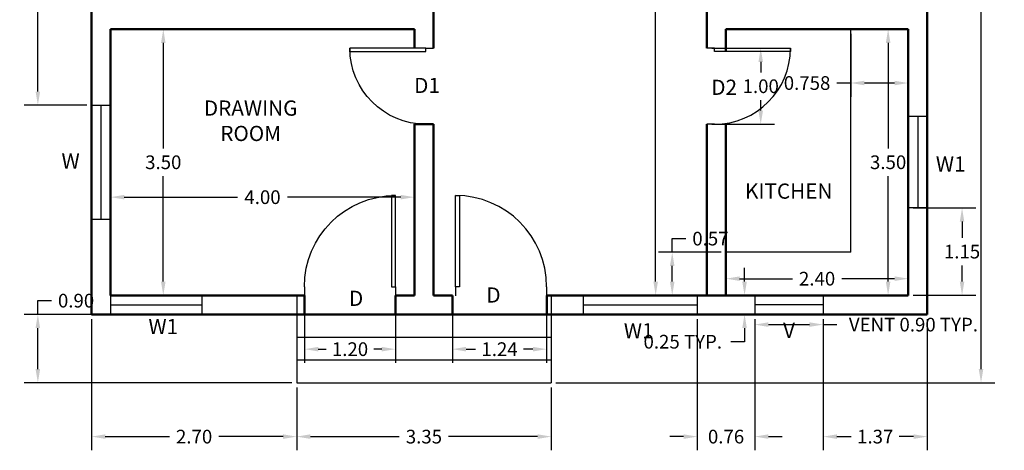
# Model space of a CAD drawing. Units: metres. Extents: x 136 to 273, y 211 to 430.
# Tile 1 of 2: x 136.09 to 149.05, y 211.01 to 216.67. Entities that reach past the tile are written whole.
import ezdxf

# ---------------------------------------------------------------- set-up
doc = ezdxf.new("R2010")
doc.units = ezdxf.units.M
doc.header["$MEASUREMENT"] = 0
for name, color, linetype, lineweight in [('A-ANNO-DIMS', 7, 'Continuous', 18), ('A-ANNO-TEXT', 221, 'Continuous', 18), ('A-AREA-IDEN', 221, 'Continuous', 25), ('A-FLOR-FIXT', 8, 'Continuous', 25), ('DOOR', 240, 'Continuous', 25), ('STEPS', 131, 'Continuous', 30), ('VN', 172, 'Continuous', 25), ('WALL', 6, 'Continuous', 50), ('WD', 80, 'Continuous', 25)]:
    doc.layers.add(name, color=color, linetype=linetype, lineweight=lineweight)
doc.styles.get("Standard").update_dxf_attribs({"font": 'arial.ttf'})
doc.dimstyles.get("Standard").update_dxf_attribs({"dimtxt": 0.18, "dimasz": 0.18, "dimexe": 0.18, "dimexo": 0.0625, "dimgap": 0.09, "dimtad": 0, "dimtih": 1, "dimtoh": 1, "dimzin": 0, "dimdsep": 46, "dimtxsty": 'Standard', "dimcen": 0.09, "dimadec": 0, "dimazin": 0, "dimtfac": 1, "dimtofl": 0, "dimtmove": 0, "dimatfit": 3, "dimfxl": 1, "dimtolj": 1, "dimtzin": 0, "dimarcsym": 0})

# ---------------------------------------------------------------- blocks, each defined once
blk = doc.blocks.new('*U3')
for p, q in [((0, 0), (0, -100)), ((1000, 0), (1000, -100))]:
    blk.add_line(p, q)
blk.add_lwpolyline([(0, 0), (0, 1000), (43.75, 1000), (43.75, 0)], close=True)
blk.add_arc((0, 0), 1000, 0, 90)
blk = doc.blocks.new('*D13')
at = {"layer": 'A-ANNO-DIMS', "color": 0, "lineweight": -2, "transparency": 16777216}
for p, q in [((137.283, 213.109), (137.283, 214.518)), ((141.283, 213.109), (141.283, 214.518)), ((137.463, 214.338), (138.956, 214.338)), ((141.103, 214.338), (139.61, 214.338))]:
    blk.add_line(p, q, dxfattribs=at)
at = {"layer": 'A-ANNO-DIMS', "color": 0, "transparency": 16777216}
for points in [[(137.463, 214.368), (137.463, 214.308), (137.283, 214.338)], [(141.103, 214.368), (141.103, 214.308), (141.283, 214.338)]]:
    blk.add_solid(points, dxfattribs=at)
at = {"layer": 'Defpoints', "color": 0, "transparency": 16777216}
for p in [(137.283, 214.338), (137.283, 213.047), (141.283, 213.047)]:
    blk.add_point(p, dxfattribs=at)
at = {"layer": 'A-ANNO-DIMS', "color": 0, "transparency": 16777216, "insert": (139.283, 214.338), "char_height": 0.18, "attachment_point": 5}
blk.add_mtext('\\A1;4.00', dxfattribs=at)
blk = doc.blocks.new('*D14')
at = {"layer": 'A-ANNO-DIMS', "color": 0, "lineweight": -2, "transparency": 16777216}
for p, q in [((137.346, 216.547), (138.157, 216.547)), ((137.977, 216.367), (137.977, 214.979)), ((137.977, 213.227), (137.977, 214.615)), ((137.346, 213.047), (138.157, 213.047))]:
    blk.add_line(p, q, dxfattribs=at)
at = {"layer": 'A-ANNO-DIMS', "color": 0, "transparency": 16777216}
for points in [[(137.947, 216.367), (138.007, 216.367), (137.977, 216.547)], [(137.947, 213.227), (138.007, 213.227), (137.977, 213.047)]]:
    blk.add_solid(points, dxfattribs=at)
at = {"layer": 'Defpoints', "color": 0, "transparency": 16777216}
for p in [(137.283, 216.547), (137.283, 213.047), (137.977, 213.047)]:
    blk.add_point(p, dxfattribs=at)
at = {"layer": 'A-ANNO-DIMS', "color": 0, "transparency": 16777216, "insert": (137.977, 214.797), "char_height": 0.18, "attachment_point": 5}
blk.add_mtext('\\A1;3.50', dxfattribs=at)
blk = doc.blocks.new('*D15')
at = {"layer": 'A-ANNO-DIMS', "color": 0, "lineweight": -2, "transparency": 16777216}
for p, q in [((145.383, 213.109), (145.383, 213.446)), ((147.783, 213.109), (147.783, 213.446)), ((145.563, 213.266), (146.258, 213.266)), ((147.603, 213.266), (146.908, 213.266))]:
    blk.add_line(p, q, dxfattribs=at)
at = {"layer": 'A-ANNO-DIMS', "color": 0, "transparency": 16777216}
for points in [[(145.563, 213.296), (145.563, 213.236), (145.383, 213.266)], [(147.603, 213.296), (147.603, 213.236), (147.783, 213.266)]]:
    blk.add_solid(points, dxfattribs=at)
at = {"layer": 'Defpoints', "color": 0, "transparency": 16777216}
for p in [(145.383, 213.266), (145.383, 213.047), (147.783, 213.047)]:
    blk.add_point(p, dxfattribs=at)
at = {"layer": 'A-ANNO-DIMS', "color": 0, "transparency": 16777216, "insert": (146.583, 213.266), "char_height": 0.18, "attachment_point": 5}
blk.add_mtext('\\A1;2.40', dxfattribs=at)
blk = doc.blocks.new('*D16')
at = {"layer": 'A-ANNO-DIMS', "color": 0, "lineweight": -2, "transparency": 16777216}
for p, q in [((147.721, 216.547), (147.338, 216.547)), ((147.518, 216.367), (147.518, 214.979)), ((147.518, 213.227), (147.518, 214.615)), ((147.721, 213.047), (147.338, 213.047))]:
    blk.add_line(p, q, dxfattribs=at)
at = {"layer": 'A-ANNO-DIMS', "color": 0, "transparency": 16777216}
for points in [[(147.488, 216.367), (147.548, 216.367), (147.518, 216.547)], [(147.488, 213.227), (147.548, 213.227), (147.518, 213.047)]]:
    blk.add_solid(points, dxfattribs=at)
at = {"layer": 'Defpoints', "color": 0, "transparency": 16777216}
for p in [(147.783, 216.547), (147.518, 213.047), (147.783, 213.047)]:
    blk.add_point(p, dxfattribs=at)
at = {"layer": 'A-ANNO-DIMS', "color": 0, "transparency": 16777216, "insert": (147.518, 214.797), "char_height": 0.18, "attachment_point": 5}
blk.add_mtext('\\A1;3.50', dxfattribs=at)
blk = doc.blocks.new('*D24')
at = {"layer": 'A-ANNO-DIMS', "color": 0, "lineweight": -2, "transparency": 16777216}
for p, q in [((144.521, 221.197), (144.638, 221.197)), ((144.458, 221.017), (144.458, 217.304)), ((144.458, 213.227), (144.458, 216.94)), ((144.521, 213.047), (144.638, 213.047))]:
    blk.add_line(p, q, dxfattribs=at)
at = {"layer": 'A-ANNO-DIMS', "color": 0, "transparency": 16777216}
for points in [[(144.428, 221.017), (144.488, 221.017), (144.458, 221.197)], [(144.428, 213.227), (144.488, 213.227), (144.458, 213.047)]]:
    blk.add_solid(points, dxfattribs=at)
at = {"layer": 'Defpoints', "color": 0, "transparency": 16777216}
for p in [(144.458, 221.197), (144.458, 213.047), (144.458, 213.047)]:
    blk.add_point(p, dxfattribs=at)
at = {"layer": 'A-ANNO-DIMS', "color": 0, "transparency": 16777216, "insert": (144.458, 217.122), "char_height": 0.18, "attachment_point": 5}
blk.add_mtext('\\A1;8.15', dxfattribs=at)
blk = doc.blocks.new('WIN-1200')
for p, q in [((0, 0), (0, 0.25)), ((1.2, 0), (1.2, 0.25)), ((1.2, 0.125), (0, 0.125))]:
    blk.add_line(p, q)
blk = doc.blocks.new('WIN-1500')
for p, q in [((0, 0), (0, 0.25)), ((1.5, 0), (1.5, 0.25)), ((1.5, 0.125), (0, 0.125))]:
    blk.add_line(p, q)
blk = doc.blocks.new('VENT-900')
for p, q in [((0, 0.9), (0.25, 0.9)), ((0.125, 0.9), (0.125, 0)), ((0, 0), (0.25, 0))]:
    blk.add_line(p, q)
blk = doc.blocks.new('*D32')
at = {"layer": 'A-ANNO-DIMS', "color": 0, "lineweight": -2, "transparency": 16777216}
for p, q in [((145.763, 212.734), (145.763, 212.482)), ((146.663, 212.734), (146.663, 212.482)), ((145.943, 212.662), (146.483, 212.662)), ((146.663, 212.662), (146.843, 212.662))]:
    blk.add_line(p, q, dxfattribs=at)
at = {"layer": 'A-ANNO-DIMS', "color": 0, "transparency": 16777216}
for points in [[(145.943, 212.692), (145.943, 212.632), (145.763, 212.662)], [(146.483, 212.692), (146.483, 212.632), (146.663, 212.662)]]:
    blk.add_solid(points, dxfattribs=at)
at = {"layer": 'Defpoints', "color": 0, "transparency": 16777216}
for p in [(145.763, 212.797), (146.663, 212.797), (146.663, 212.662)]:
    blk.add_point(p, dxfattribs=at)
at = {"layer": 'A-ANNO-DIMS', "color": 0, "transparency": 16777216, "insert": (147.851, 212.662), "char_height": 0.18, "attachment_point": 5}
blk.add_mtext('\\A1;VENT 0.90 TYP.', dxfattribs=at)
blk = doc.blocks.new('*D33')
at = {"layer": 'A-ANNO-DIMS', "color": 0, "lineweight": -2, "transparency": 16777216}
for p, q in [((145.628, 213.227), (145.628, 213.407)), ((145.701, 213.047), (145.448, 213.047)), ((145.701, 212.797), (145.448, 212.797)), ((145.628, 212.617), (145.628, 212.437)), ((145.628, 212.437), (145.448, 212.437))]:
    blk.add_line(p, q, dxfattribs=at)
at = {"layer": 'A-ANNO-DIMS', "color": 0, "transparency": 16777216}
for points in [[(145.598, 213.227), (145.658, 213.227), (145.628, 213.047)], [(145.598, 212.617), (145.658, 212.617), (145.628, 212.797)]]:
    blk.add_solid(points, dxfattribs=at)
at = {"layer": 'Defpoints', "color": 0, "transparency": 16777216}
for p in [(145.763, 213.047), (145.628, 212.797), (145.763, 212.797)]:
    blk.add_point(p, dxfattribs=at)
at = {"layer": 'A-ANNO-DIMS', "color": 0, "transparency": 16777216, "insert": (144.815, 212.437), "char_height": 0.18, "attachment_point": 5}
blk.add_mtext('\\A1;0.25 TYP.', dxfattribs=at)
blk = doc.blocks.new('*D35')
at = {"layer": 'A-ANNO-DIMS', "color": 0, "lineweight": -2, "transparency": 16777216}
for p, q in [((148.096, 225.297), (148.921, 225.297)), ((148.741, 225.117), (148.741, 218.779)), ((148.741, 212.077), (148.741, 218.415)), ((143.146, 211.897), (148.921, 211.897))]:
    blk.add_line(p, q, dxfattribs=at)
at = {"layer": 'A-ANNO-DIMS', "color": 0, "transparency": 16777216}
for points in [[(148.711, 225.117), (148.771, 225.117), (148.741, 225.297)], [(148.711, 212.077), (148.771, 212.077), (148.741, 211.897)]]:
    blk.add_solid(points, dxfattribs=at)
at = {"layer": 'Defpoints', "color": 0, "transparency": 16777216}
for p in [(148.033, 225.297), (148.741, 225.297), (143.083, 211.897)]:
    blk.add_point(p, dxfattribs=at)
at = {"layer": 'A-ANNO-DIMS', "color": 0, "transparency": 16777216, "insert": (148.741, 218.597), "char_height": 0.18, "attachment_point": 5}
blk.add_mtext('\\A1;13.40', dxfattribs=at)
blk = doc.blocks.new('*D36')
at = {"layer": 'A-ANNO-DIMS', "color": 0, "lineweight": -2, "transparency": 16777216}
for p, q in [((136.326, 212.797), (136.326, 212.977)), ((136.326, 212.977), (136.506, 212.977)), ((139.671, 212.797), (136.146, 212.797)), ((136.326, 212.077), (136.326, 212.617)), ((139.671, 211.897), (136.146, 211.897))]:
    blk.add_line(p, q, dxfattribs=at)
at = {"layer": 'A-ANNO-DIMS', "color": 0, "transparency": 16777216}
for points in [[(136.296, 212.617), (136.356, 212.617), (136.326, 212.797)], [(136.296, 212.077), (136.356, 212.077), (136.326, 211.897)]]:
    blk.add_solid(points, dxfattribs=at)
at = {"layer": 'Defpoints', "color": 0, "transparency": 16777216}
for p in [(136.326, 212.797), (139.733, 212.797), (139.733, 211.897)]:
    blk.add_point(p, dxfattribs=at)
at = {"layer": 'A-ANNO-DIMS', "color": 0, "transparency": 16777216, "insert": (136.829, 212.977), "char_height": 0.18, "attachment_point": 5}
blk.add_mtext('\\A1;0.90', dxfattribs=at)
blk = doc.blocks.new('*D37')
at = {"layer": 'A-ANNO-DIMS', "color": 0, "lineweight": -2, "transparency": 16777216}
for p, q in [((139.733, 211.834), (139.733, 211.009)), ((143.083, 211.834), (143.083, 211.009)), ((139.913, 211.189), (141.084, 211.189)), ((142.903, 211.189), (141.732, 211.189))]:
    blk.add_line(p, q, dxfattribs=at)
at = {"layer": 'A-ANNO-DIMS', "color": 0, "transparency": 16777216}
for points in [[(139.913, 211.219), (139.913, 211.159), (139.733, 211.189)], [(142.903, 211.219), (142.903, 211.159), (143.083, 211.189)]]:
    blk.add_solid(points, dxfattribs=at)
at = {"layer": 'Defpoints', "color": 0, "transparency": 16777216}
for p in [(139.733, 211.897), (143.083, 211.897), (143.083, 211.189)]:
    blk.add_point(p, dxfattribs=at)
at = {"layer": 'A-ANNO-DIMS', "color": 0, "transparency": 16777216, "insert": (141.408, 211.189), "char_height": 0.18, "attachment_point": 5}
blk.add_mtext('\\A1;3.35', dxfattribs=at)
blk = doc.blocks.new('*D38')
at = {"layer": 'A-ANNO-DIMS', "color": 0, "lineweight": -2, "transparency": 16777216}
for p, q in [((137.033, 212.734), (137.033, 211.009)), ((139.733, 211.834), (139.733, 211.009)), ((137.213, 211.189), (138.058, 211.189)), ((139.553, 211.189), (138.708, 211.189))]:
    blk.add_line(p, q, dxfattribs=at)
at = {"layer": 'A-ANNO-DIMS', "color": 0, "transparency": 16777216}
for points in [[(137.213, 211.219), (137.213, 211.159), (137.033, 211.189)], [(139.553, 211.219), (139.553, 211.159), (139.733, 211.189)]]:
    blk.add_solid(points, dxfattribs=at)
at = {"layer": 'Defpoints', "color": 0, "transparency": 16777216}
for p in [(137.033, 212.797), (139.733, 211.897), (139.733, 211.189)]:
    blk.add_point(p, dxfattribs=at)
at = {"layer": 'A-ANNO-DIMS', "color": 0, "transparency": 16777216, "insert": (138.383, 211.189), "char_height": 0.18, "attachment_point": 5}
blk.add_mtext('\\A1;2.70', dxfattribs=at)
blk = doc.blocks.new('*D43')
at = {"layer": 'A-ANNO-DIMS', "color": 0, "lineweight": -2, "transparency": 16777216}
for p, q in [((136.971, 218.397), (136.146, 218.397)), ((136.326, 218.217), (136.326, 217.154)), ((136.326, 215.727), (136.326, 216.79)), ((136.971, 215.547), (136.146, 215.547))]:
    blk.add_line(p, q, dxfattribs=at)
at = {"layer": 'A-ANNO-DIMS', "color": 0, "transparency": 16777216}
for points in [[(136.296, 218.217), (136.356, 218.217), (136.326, 218.397)], [(136.296, 215.727), (136.356, 215.727), (136.326, 215.547)]]:
    blk.add_solid(points, dxfattribs=at)
at = {"layer": 'Defpoints', "color": 0, "transparency": 16777216}
for p in [(136.326, 218.397), (137.033, 218.397), (137.033, 215.547)]:
    blk.add_point(p, dxfattribs=at)
at = {"layer": 'A-ANNO-DIMS', "color": 0, "transparency": 16777216, "insert": (136.326, 216.972), "char_height": 0.18, "attachment_point": 5}
blk.add_mtext('\\A1;2.85', dxfattribs=at)
blk = doc.blocks.new('*D44')
at = {"layer": 'A-ANNO-DIMS', "color": 0, "lineweight": -2, "transparency": 16777216}
for p, q in [((147.846, 214.197), (148.671, 214.197)), ((148.491, 214.017), (148.491, 213.804)), ((148.491, 213.227), (148.491, 213.44)), ((147.846, 213.047), (148.671, 213.047))]:
    blk.add_line(p, q, dxfattribs=at)
at = {"layer": 'A-ANNO-DIMS', "color": 0, "transparency": 16777216}
for points in [[(148.461, 214.017), (148.521, 214.017), (148.491, 214.197)], [(148.461, 213.227), (148.521, 213.227), (148.491, 213.047)]]:
    blk.add_solid(points, dxfattribs=at)
at = {"layer": 'Defpoints', "color": 0, "transparency": 16777216}
for p in [(147.783, 214.197), (147.783, 213.047), (148.491, 213.047)]:
    blk.add_point(p, dxfattribs=at)
at = {"layer": 'A-ANNO-DIMS', "color": 0, "transparency": 16777216, "insert": (148.491, 213.622), "char_height": 0.18, "attachment_point": 5}
blk.add_mtext('\\A1;1.15', dxfattribs=at)
blk = doc.blocks.new('*D46')
at = {"layer": 'A-ANNO-DIMS', "color": 0, "lineweight": -2, "transparency": 16777216}
for p, q in [((146.663, 212.734), (146.663, 211.009)), ((148.033, 212.734), (148.033, 211.009)), ((146.843, 211.189), (147.033, 211.189)), ((147.853, 211.189), (147.663, 211.189))]:
    blk.add_line(p, q, dxfattribs=at)
at = {"layer": 'A-ANNO-DIMS', "color": 0, "transparency": 16777216}
for points in [[(146.843, 211.219), (146.843, 211.159), (146.663, 211.189)], [(147.853, 211.219), (147.853, 211.159), (148.033, 211.189)]]:
    blk.add_solid(points, dxfattribs=at)
at = {"layer": 'Defpoints', "color": 0, "transparency": 16777216}
for p in [(146.663, 212.797), (148.033, 212.797), (148.033, 211.189)]:
    blk.add_point(p, dxfattribs=at)
at = {"layer": 'A-ANNO-DIMS', "color": 0, "transparency": 16777216, "insert": (147.348, 211.189), "char_height": 0.18, "attachment_point": 5}
blk.add_mtext('\\A1;1.37', dxfattribs=at)
blk = doc.blocks.new('*D47')
at = {"layer": 'A-ANNO-DIMS', "color": 0, "lineweight": -2, "transparency": 16777216}
for p, q in [((145.005944, 212.734143), (145.005944, 211.009143)), ((145.763332, 212.734143), (145.763332, 211.009143)), ((144.825944, 211.189143), (144.645944, 211.189143)), ((145.943332, 211.189143), (146.123332, 211.189143))]:
    blk.add_line(p, q, dxfattribs=at)
at = {"layer": 'A-ANNO-DIMS', "color": 0, "transparency": 16777216}
for points in [[(144.825944, 211.219143), (144.825944, 211.159143), (145.005944, 211.189143)], [(145.943332, 211.219143), (145.943332, 211.159143), (145.763332, 211.189143)]]:
    blk.add_solid(points, dxfattribs=at)
at = {"layer": 'Defpoints', "color": 0, "transparency": 16777216}
for p in [(145.005944, 212.796643), (145.763332, 212.796643), (145.763332, 211.189143)]:
    blk.add_point(p, dxfattribs=at)
at = {"layer": 'A-ANNO-DIMS', "color": 0, "transparency": 16777216, "insert": (145.384638, 211.189143), "char_height": 0.18, "attachment_point": 5}
blk.add_mtext('\\A1;0.76', dxfattribs=at)
blk = doc.blocks.new('*D48')
at = {"layer": 'A-ANNO-DIMS', "color": 0, "lineweight": -2, "transparency": 16777216}
for p, q in [((139.837, 212.984), (139.837, 212.159)), ((141.033, 212.984), (141.033, 212.159)), ((140.017, 212.339), (140.12, 212.339)), ((140.853, 212.339), (140.75, 212.339))]:
    blk.add_line(p, q, dxfattribs=at)
at = {"layer": 'A-ANNO-DIMS', "color": 0, "transparency": 16777216}
for points in [[(140.017, 212.369), (140.017, 212.309), (139.837, 212.339)], [(140.853, 212.369), (140.853, 212.309), (141.033, 212.339)]]:
    blk.add_solid(points, dxfattribs=at)
at = {"layer": 'Defpoints', "color": 0, "transparency": 16777216}
for p in [(139.837, 213.047), (141.033, 213.047), (139.837, 212.339)]:
    blk.add_point(p, dxfattribs=at)
at = {"layer": 'A-ANNO-DIMS', "color": 0, "transparency": 16777216, "insert": (140.435, 212.339), "char_height": 0.18, "attachment_point": 5}
blk.add_mtext('\\A1;1.20', dxfattribs=at)
blk = doc.blocks.new('*D49')
at = {"layer": 'A-ANNO-DIMS', "color": 0, "lineweight": -2, "transparency": 16777216}
for p, q in [((141.783, 212.984), (141.783, 212.159)), ((143.022, 212.984), (143.022, 212.159)), ((141.963, 212.339), (142.088, 212.339)), ((142.842, 212.339), (142.718, 212.339))]:
    blk.add_line(p, q, dxfattribs=at)
at = {"layer": 'A-ANNO-DIMS', "color": 0, "transparency": 16777216}
for points in [[(141.963, 212.369), (141.963, 212.309), (141.783, 212.339)], [(142.842, 212.369), (142.842, 212.309), (143.022, 212.339)]]:
    blk.add_solid(points, dxfattribs=at)
at = {"layer": 'Defpoints', "color": 0, "transparency": 16777216}
for p in [(141.783, 213.047), (143.022, 213.047), (141.783, 212.339)]:
    blk.add_point(p, dxfattribs=at)
at = {"layer": 'A-ANNO-DIMS', "color": 0, "transparency": 16777216, "insert": (142.403, 212.339), "char_height": 0.18, "attachment_point": 5}
blk.add_mtext('\\A1;1.24', dxfattribs=at)
blk = doc.blocks.new('*D55')
at = {"layer": 'A-ANNO-DIMS', "color": 0, "lineweight": -2, "transparency": 16777216}
for p, q in [((145.196, 216.297), (146.021, 216.297)), ((145.841, 216.117), (145.841, 215.979)), ((145.841, 215.477), (145.841, 215.615)), ((145.196, 215.297), (146.021, 215.297))]:
    blk.add_line(p, q, dxfattribs=at)
at = {"layer": 'A-ANNO-DIMS', "color": 0, "transparency": 16777216}
for points in [[(145.811, 216.117), (145.871, 216.117), (145.841, 216.297)], [(145.811, 215.477), (145.871, 215.477), (145.841, 215.297)]]:
    blk.add_solid(points, dxfattribs=at)
at = {"layer": 'Defpoints', "color": 0, "transparency": 16777216}
for p in [(145.133, 216.297), (145.133, 215.297), (145.841, 215.297)]:
    blk.add_point(p, dxfattribs=at)
at = {"layer": 'A-ANNO-DIMS', "color": 0, "transparency": 16777216, "insert": (145.841, 215.797), "char_height": 0.18, "attachment_point": 5}
blk.add_mtext('\\A1;1.00', dxfattribs=at)
blk = doc.blocks.new('*D56')
at = {"layer": 'A-ANNO-DIMS', "color": 0, "lineweight": -2, "transparency": 16777216}
for p, q in [((144.676, 213.613), (144.676, 213.793)), ((144.676, 213.793), (144.856, 213.793)), ((145.321, 213.613), (144.496, 213.613)), ((144.676, 213.227), (144.676, 213.433)), ((145.321, 213.047), (144.496, 213.047))]:
    blk.add_line(p, q, dxfattribs=at)
at = {"layer": 'A-ANNO-DIMS', "color": 0, "transparency": 16777216}
for points in [[(144.646, 213.433), (144.706, 213.433), (144.676, 213.613)], [(144.646, 213.227), (144.706, 213.227), (144.676, 213.047)]]:
    blk.add_solid(points, dxfattribs=at)
at = {"layer": 'Defpoints', "color": 0, "transparency": 16777216}
for p in [(144.676, 213.613), (145.383, 213.613), (145.383, 213.047)]:
    blk.add_point(p, dxfattribs=at)
at = {"layer": 'A-ANNO-DIMS', "color": 0, "transparency": 16777216, "insert": (145.179, 213.793), "char_height": 0.18, "attachment_point": 5}
blk.add_mtext('\\A1;0.57', dxfattribs=at)
blk = doc.blocks.new('*D57')
at = {"layer": 'A-ANNO-DIMS', "color": 0, "lineweight": -2, "transparency": 16777216}
for p, q in [((147.025, 216.484), (147.025, 215.659)), ((147.783, 216.484), (147.783, 215.659)), ((147.025, 215.839), (146.845, 215.839)), ((147.603, 215.839), (147.205, 215.839))]:
    blk.add_line(p, q, dxfattribs=at)
at = {"layer": 'A-ANNO-DIMS', "color": 0, "transparency": 16777216}
for points in [[(147.205, 215.869), (147.205, 215.809), (147.025, 215.839)], [(147.603, 215.869), (147.603, 215.809), (147.783, 215.839)]]:
    blk.add_solid(points, dxfattribs=at)
at = {"layer": 'Defpoints', "color": 0, "transparency": 16777216}
for p in [(147.025, 216.547), (147.783, 216.547), (147.025, 215.839)]:
    blk.add_point(p, dxfattribs=at)
at = {"layer": 'A-ANNO-DIMS', "color": 0, "transparency": 16777216, "insert": (146.451, 215.839), "char_height": 0.18, "attachment_point": 5}
blk.add_mtext('\\A1;0.758', dxfattribs=at)

msp = doc.modelspace()

# ---------------------------------------------------------------- linework, layer by layer
at = {"layer": 'A-FLOR-FIXT'}
for q in [(147.025, 216.5466), (145.383, 213.6132)]:
    msp.add_line((147.025, 213.6132), q, dxfattribs=at)
at = {"layer": 'STEPS'}
for p, q in [((139.733, 213.0466), (139.733, 212.7966)), ((143.083, 213.0466), (143.083, 212.7966)), ((139.733, 212.7966), (139.733, 211.8966)), ((143.083, 212.7966), (143.083, 211.8966)), ((139.733, 212.4966), (143.083, 212.4966)), ((139.733, 212.1966), (143.083, 212.1966)), ((139.733, 211.8966), (143.083, 211.8966))]:
    msp.add_line(p, q, dxfattribs=at)
at = {"layer": 'WALL'}
for p, q in [((137.033, 221.1966), (137.033, 216.5466)), ((141.533, 220.0466), (141.533, 216.5466)), ((145.133, 218.2466), (145.133, 216.5466)), ((148.033, 217.9966), (148.033, 216.5466)), ((137.033, 216.5466), (137.033, 212.7966)), ((141.283, 216.5466), (137.283, 216.5466)), ((137.283, 216.5466), (137.283, 213.0466)), ((141.283, 216.5466), (141.283, 216.2966)), ((141.533, 216.5466), (141.533, 216.2966)), ((145.133, 216.5466), (145.133, 216.2966)), ((145.133, 216.5466), (145.133, 216.2966)), ((145.383, 216.5466), (147.783, 216.5466)), ((145.383, 216.5466), (145.383, 216.2529)), ((145.383, 216.5466), (145.383, 216.2529)), ((147.783, 216.5466), (147.783, 213.0466)), ((148.033, 216.5466), (148.033, 212.7966)), ((141.533, 215.2966), (141.283, 215.2966)), ((141.283, 215.2966), (141.283, 213.0466)), ((141.533, 215.2966), (141.533, 213.0466)), ((145.133, 215.2966), (145.133, 213.0466)), ((145.383, 215.308), (145.383, 213.0466)), ((139.8372, 213.0466), (137.283, 213.0466)), ((139.8372, 213.0466), (139.8372, 212.7966)), ((141.283, 213.0466), (141.033, 213.0466)), ((141.033, 213.0466), (141.033, 212.7966)), ((141.533, 213.0466), (141.783, 213.0466)), ((141.783, 213.0466), (141.783, 212.7966)), ((143.0224, 213.0466), (147.783, 213.0466)), ((143.0239, 213.0466), (143.0239, 212.7966)), ((140.033, 212.7966), (137.033, 212.7966)), ((141.533, 212.7966), (140.033, 212.7966)), ((141.533, 212.7966), (142.783, 212.7966)), ((142.783, 212.7966), (148.033, 212.7966))]:
    msp.add_line(p, q, dxfattribs=at)

# ---------------------------------------------------------------- block references
at = {"layer": 'DOOR', "yscale": 0.001, "zscale": 0.001}
for p, xscale, rotation in [((141.433, 216.2966), -0.001, 90), ((145.233, 216.2966), 0.001, 270)]:
    msp.add_blockref('*U3', p, dxfattribs=dict(at, xscale=xscale, rotation=rotation))
at = {"layer": 'DOOR', "yscale": 0.0011992359422906, "zscale": 0.0011992359422906}
for p, xscale in [((141.033, 213.1606), -0.0011992359422906), ((141.8231, 213.1606), 0.0011992359422906)]:
    msp.add_blockref('*U3', p, dxfattribs=dict(at, xscale=xscale))
at = {"layer": 'VN', "rotation": 270.0000000000009}
msp.add_blockref('VENT-900', (145.7633, 213.0466), dxfattribs=at)
at = {"layer": 'WD'}
for name, p, rotation in [('WIN-1500', (137.033, 215.5466), 270.0000000000042), ('WIN-1200', (148.033, 214.1966), 90), ('WIN-1200', (138.483, 213.0466), 180), ('WIN-1500', (145.0059, 213.0466), 180)]:
    msp.add_blockref(name, p, dxfattribs=dict(at, rotation=rotation))

# ---------------------------------------------------------------- texts
at = {"layer": 'A-ANNO-TEXT', "char_height": 0.2, "attachment_point": 1}
for s, width, insert in [('D1  ', 0.276534, (141.2792, 215.9071)), ('D2  ', 0.276534, (145.1904, 215.883)), ('W ', 2.156428, (136.6375, 214.9132)), ('W1 ', 0.406895, (148.1459, 214.8738)), ('D  ', 0.276534, (140.422, 213.1074)), ('\\pxqc;D  ', 0.276534, (142.1855, 213.1511)), ('W1 ', 0.406895, (137.7817, 212.7367)), ('W1 ', 0.406895, (144.0389, 212.6809)), ('V ', 0.604517, (146.1346, 212.6867))]:
    msp.add_mtext_dynamic_manual_height_columns(s, width=width, gutter_width=1, heights=[0], dxfattribs=dict(at, insert=insert))
at = {"layer": 'A-AREA-IDEN', "char_height": 0.2, "attachment_point": 1}
for s, width, insert in [('\\pxqc;DRAWING ROOM', 1.029881, (138.6122, 215.6093)), ('\\pxqc;KITCHEN', 1.372303, (145.5235, 214.5177))]:
    msp.add_mtext_dynamic_manual_height_columns(s, width=width, gutter_width=1, heights=[0], dxfattribs=dict(at, insert=insert))

# ---------------------------------------------------------------- dimensions: what is measured, and where the dimension line sits
at = {"layer": 'A-ANNO-DIMS'}
for base, p1, p2, angle, override, picture, middle in [((148.7405, 225.2966), (143.083, 211.8966), (148.033, 225.2966), 90, {"dimdec": 2, "dimlfac": 1, "dimrnd": 0, "dimzin": 0, "dimdsep": 46, "dimlunit": 2}, '*D35', (148.7405, 218.5966)), ((144.458, 213.0466), (144.458, 221.1966), (144.458, 213.0466), 90, {"dimclrd": 0, "dimclre": 0, "dimclrt": 0}, '*D24', (144.458, 217.1216)), ((136.3255, 218.3966), (137.033, 215.5466), (137.033, 218.3966), 90, {"dimdec": 2, "dimlfac": 1, "dimrnd": 0, "dimzin": 0, "dimdsep": 46, "dimlunit": 2}, '*D43', (136.3255, 216.9716)), ((137.9768, 213.0466), (137.283, 216.5466), (137.283, 213.0466), 90, {"dimclrd": 0, "dimclre": 0, "dimclrt": 0}, '*D14', (137.9768, 214.7966)), ((147.025, 215.8391), (147.783, 216.5466), (147.025, 216.5466), 180, {"dimdec": 3, "dimlfac": 1, "dimrnd": 0, "dimzin": 0, "dimdsep": 46, "dimlunit": 2}, '*D57', (146.4511, 215.8391)), ((145.8405, 215.2966), (145.133, 216.2966), (145.133, 215.2966), 270, {"dimdec": 2, "dimlfac": 1, "dimrnd": 0, "dimzin": 0, "dimdsep": 46, "dimlunit": 2}, '*D55', (145.8405, 215.7966)), ((148.4905, 213.0466), (147.783, 214.1966), (147.783, 213.0466), 270, {"dimdec": 2, "dimlfac": 1, "dimrnd": 0, "dimzin": 0, "dimdsep": 46, "dimlunit": 2}, '*D44', (148.4905, 213.6216)), ((144.6755, 213.6132), (145.383, 213.0466), (145.383, 213.6132), 90, {"dimdec": 2, "dimlfac": 1, "dimrnd": 0, "dimzin": 0, "dimdsep": 46, "dimlunit": 2}, '*D56', (145.1793, 213.7932)), ((136.3255, 212.7966), (139.733, 211.8966), (139.733, 212.7966), 90, {"dimdec": 2, "dimlfac": 1, "dimrnd": 0, "dimzin": 0, "dimdsep": 46, "dimlunit": 2}, '*D36', (136.829, 212.9766)), ((139.8372, 212.3391), (141.033, 213.0466), (139.8372, 213.0466), 180, {"dimdec": 2, "dimlfac": 1, "dimrnd": 0, "dimzin": 0, "dimdsep": 46, "dimlunit": 2}, '*D48', (140.4351, 212.3391)), ((141.783, 212.3391), (143.0224, 213.0466), (141.783, 213.0466), 180, {"dimdec": 2, "dimlfac": 1, "dimrnd": 0, "dimzin": 0, "dimdsep": 46, "dimlunit": 2}, '*D49', (142.4027, 212.3391))]:
    dim = msp.add_linear_dim(base=base, p1=p1, p2=p2, angle=angle, dimstyle='Standard', override=override, dxfattribs=at)
    dim.commit()
    dim.dimension.update_dxf_attribs({"geometry": picture, "text_midpoint": middle})
dim = msp.add_linear_dim(base=(147.5181, 213.0466), p1=(147.783, 216.5466), p2=(147.783, 213.0466), angle=90, dimstyle='Standard', override={"dimclrd": 0, "dimclre": 0, "dimclrt": 0}, dxfattribs=at)
dim.commit()
dim.dimension.update_dxf_attribs({"geometry": '*D16', "text_midpoint": (147.5181, 214.7966), "dimtype": 160})
dim = msp.add_linear_dim(base=(137.283, 214.3378), p1=(141.283, 213.0466), p2=(137.283, 213.0466), dimstyle='Standard', override={"dimclrd": 0, "dimclre": 0, "dimclrt": 0}, dxfattribs=at)
dim.commit()
dim.dimension.update_dxf_attribs({"geometry": '*D13', "text_midpoint": (139.283, 214.3378), "dimtype": 160})
for base, p1, p2, angle, text, picture, middle in [((145.6283, 212.7966), (145.7633, 213.0466), (145.7633, 212.7966), 270, '<> TYP.', '*D33', (144.8154, 212.4366)), ((146.6633, 212.6616), (145.7633, 212.7966), (146.6633, 212.7966), 0, 'VENT <> TYP.', '*D32', (147.8512, 212.6616))]:
    dim = msp.add_linear_dim(base=base, p1=p1, p2=p2, angle=angle, text=text, dimstyle='Standard', override={"dimdec": 2, "dimlfac": 1, "dimrnd": 0, "dimzin": 0, "dimdsep": 46, "dimlunit": 2}, dxfattribs=at)
    dim.commit()
    dim.dimension.update_dxf_attribs({"geometry": picture, "text_midpoint": middle})
for base, p1, p2, override, picture, middle in [((145.383, 213.2655), (147.783, 213.0466), (145.383, 213.0466), {"dimclrd": 0, "dimclre": 0, "dimclrt": 0}, '*D15', (146.583, 213.2655)), ((139.733, 211.1891), (137.033, 212.7966), (139.733, 211.8966), {"dimdec": 2, "dimlfac": 1, "dimrnd": 0, "dimzin": 0, "dimdsep": 46, "dimlunit": 2}, '*D38', (138.383, 211.1891)), ((145.7633, 211.1891), (145.0059, 212.7966), (145.7633, 212.7966), {"dimdec": 2, "dimlfac": 1, "dimrnd": 0, "dimzin": 0, "dimdsep": 46, "dimlunit": 2}, '*D47', (145.3846, 211.1891)), ((148.033, 211.1891), (146.6633, 212.7966), (148.033, 212.7966), {"dimdec": 2, "dimlfac": 1, "dimrnd": 0, "dimzin": 0, "dimdsep": 46, "dimlunit": 2}, '*D46', (147.3482, 211.1891)), ((143.083, 211.1891), (139.733, 211.8966), (143.083, 211.8966), {"dimdec": 2, "dimlfac": 1, "dimrnd": 0, "dimzin": 0, "dimdsep": 46, "dimlunit": 2}, '*D37', (141.408, 211.1891))]:
    dim = msp.add_linear_dim(base=base, p1=p1, p2=p2, dimstyle='Standard', override=override, dxfattribs=at)
    dim.commit()
    dim.dimension.update_dxf_attribs({"geometry": picture, "text_midpoint": middle})

doc.saveas('drawing.dxf')
